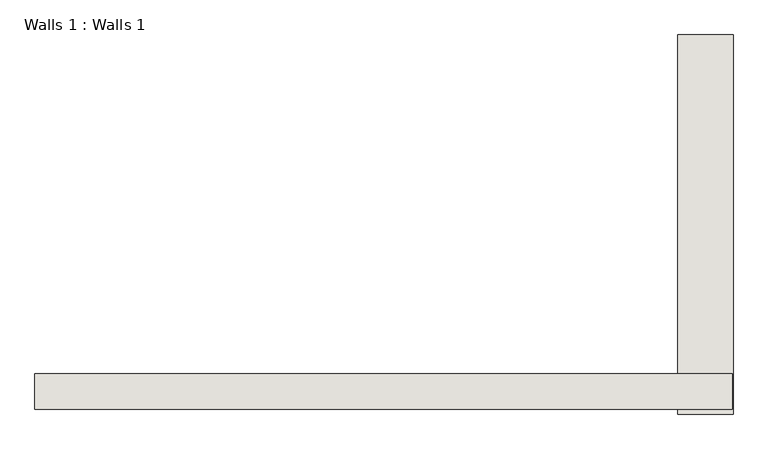
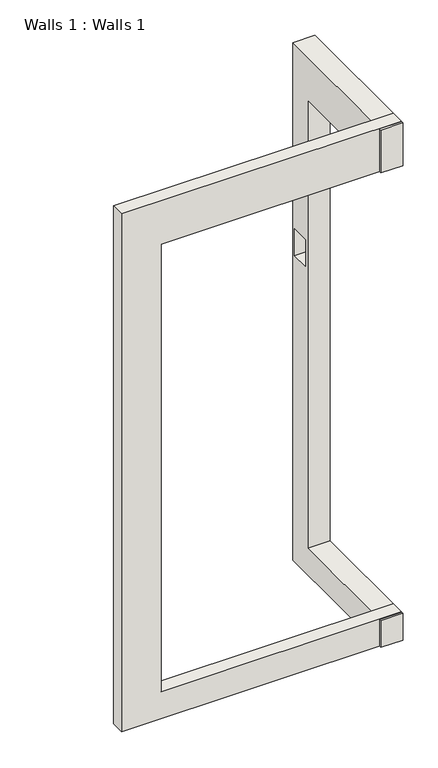
"""IFC4 building model written with IfcOpenShell, lengths in millimetres: wall geometry, Walls 1 : Walls 1."""

from ifc_helpers import new_model, si_unit, frame, origin, place, context, project, spatial, polyline, outline, extrude, source, transform, mapped, element, save


def walls_1_walls_1_fa617820(model_context):
    return source(origin(), model_context, "Body", "SweptSolid", [
        extrude(outline(polyline([(1960.0609482, 13971.7417433), (1960.0609482, 2136.0546017), (-1336.1296377, 2136.0546017), (-1336.1296377, 2745.925211), (1401.2609482, 2745.925211), (1401.2609482, 12990.4779222), (-1338.4077903, 12990.4779222), (-1338.4077903, 13971.7417433), (1960.0609482, 13971.7417433)]), holes=[polyline([(1496.1989255, 9746.9562869), (1496.1989255, 9137.3562869), (1902.5989255, 9137.3562869), (1902.5989255, 9746.9562869), (1496.1989255, 9746.9562869)])]), frame((1662.3254876, 0.0, 0.0), z_axis=(1.0, 0.0, 0.0), x_axis=(0.0, 1.0, 0.0)), (0.0, 0.0, 1.0), 479.5445618),
        extrude(outline(polyline([(13980.6021774, -3925.6745124), (2141.8917985, -3925.6745124), (2141.8917985, 2132.1075545), (2756.732239, 2132.1075545), (2756.732239, -3073.2758541), (12990.5535049, -3073.2758541), (12990.5535049, 2135.7152923), (13980.6021774, 2135.7152923), (13980.6021774, -3925.6745124)])), frame((0.0, -1291.1390518, 0.0), z_axis=(0.0, 1.0, 0.0), x_axis=(0.0, 0.0, 1.0)), (0.0, 0.0, 1.0), 304.8),
    ])


if __name__ == "__main__":
    model = new_model("IFC4")
    model_context = context("Model", 3, world=origin())
    ifc_project = project(units=[si_unit("LENGTHUNIT", "METRE", prefix="MILLI")], contexts=[model_context])
    site = spatial("IfcSite", under=ifc_project)
    building = spatial("IfcBuilding", under=site)
    placement = place(None, origin())
    walls_1_walls_1_shape = walls_1_walls_1_fa617820(model_context)
    element("IfcWall", 1, ObjectType="Walls 1 : Walls 1", at=placement, inside=building, context=model_context, shape_type="MappedRepresentation", body=[
        mapped(walls_1_walls_1_shape, transform((0.0, 0.0, 0.0), x_axis=(1.0, 0.0, 0.0), y_axis=(0.0, 1.0, 0.0), z_axis=(0.0, 0.0, 1.0))),
    ])
    save(model, "model.ifc")

# Revit data of these elements
# Element 1 (IfcWall, "Walls 1 : Walls 1")
#   Materials on its faces: "Default Wall"
# Materials
#   "Default Wall": colour RGB 128 128 128, transparency 0
